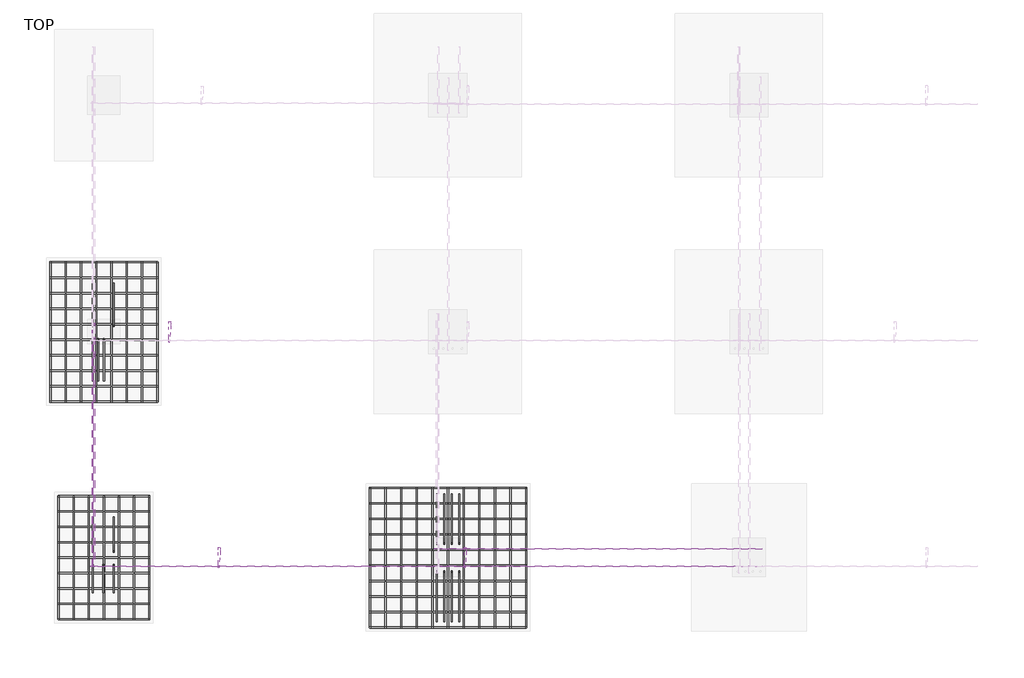
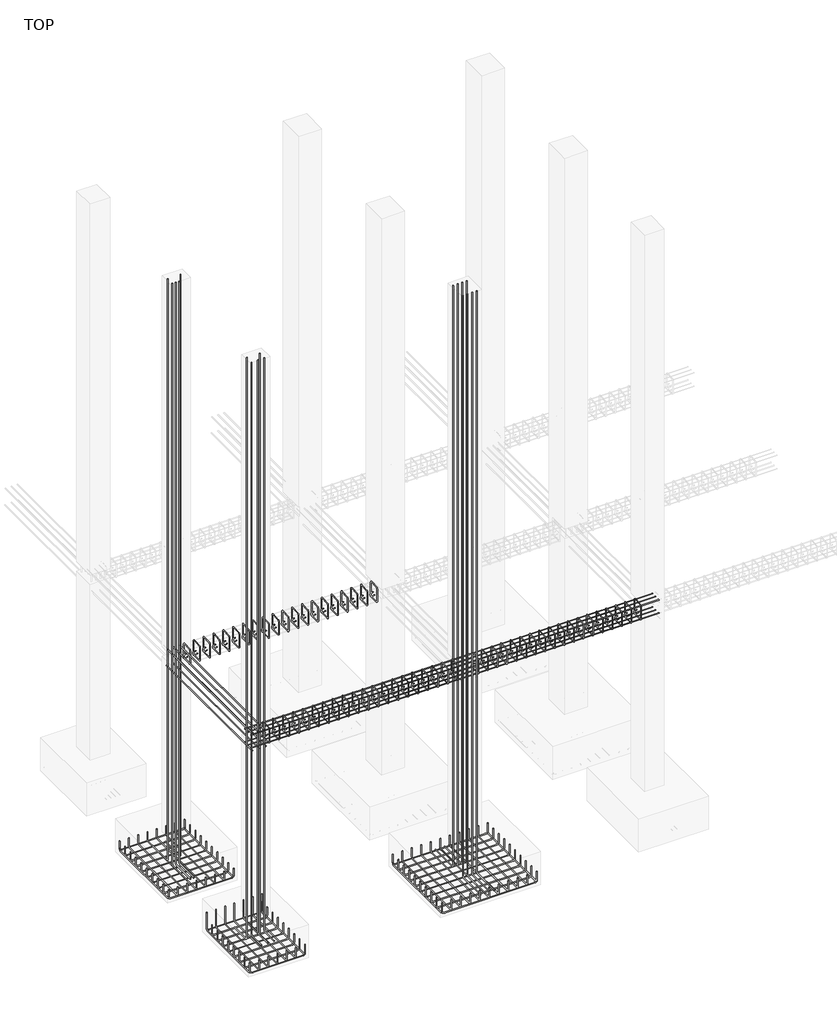
# One storey, part 2 of 8: 21 reinforcing bars.
"""IFC4 building model written with IfcOpenShell, lengths in millimetres."""

from ifc_helpers import new_model, si_unit, point, frame, origin, place, context, project, spatial, polyline, circle_curve, trimmed, segment, composite_curve, source, transform, mapped, element, save
from ifc_brep_helpers import swept_disk

model = new_model("IFC4")

# Units and contexts
model_context = context("Model", 3, world=origin())
ifc_project = project(units=[si_unit("LENGTHUNIT", "METRE", prefix="MILLI")], contexts=[model_context])

# Site, building, storey
site = spatial("IfcSite", under=ifc_project)
building = spatial("IfcBuilding", under=site)
storey = spatial("IfcBuildingStorey", under=building, Name="TOP", Elevation=0.0)

# Reinforcing bars
placement = place(None, origin())
reinforcing_bar_shape = source(origin(), model_context, "Body", "SolidModel", [
    swept_disk(composite_curve([segment(polyline([(-4743.7160601, 1689.3463601, -206.0605272), (-4743.7160601, 1689.3463601, -467.4)]), True, "CONTINUOUS"), segment(trimmed(circle_curve(frame((-4743.7160601, 1659.3463601, -467.4), z_axis=(-1.0, 0.0, 0.0), x_axis=(0.0, 30.0, 0.0)), 30.0), [point((-4743.7160601, 1689.3463601, -467.4))], [point((-4743.7160601, 1659.3463601, -497.4))], True, "CARTESIAN"), True, "CONTINUOUS"), segment(polyline([(-4743.7160601, 1659.3463601, -497.4), (-4743.7160601, 577.5307576, -497.4)]), True, "CONTINUOUS"), segment(trimmed(circle_curve(frame((-4743.7160601, 577.5307576, -467.4), z_axis=(-1.0, 0.0, 0.0), x_axis=(0.0, 0.0, -30.0)), 30.0), [point((-4743.7160601, 577.5307576, -497.4))], [point((-4743.7160601, 547.5307576, -467.4))], True, "CARTESIAN"), True, "CONTINUOUS"), segment(polyline([(-4743.7160601, 547.5307576, -467.4), (-4743.7160601, 547.5307576, -331.0)]), True, "CONTINUOUS")], self_intersect=False), 6.0),
])
element("IfcReinforcingBar", 1, at=placement, inside=storey, context=model_context, shape_type="MappedRepresentation", body=[
    mapped(reinforcing_bar_shape, transform((0.0, 0.0, 0.0), x_axis=(1.0, 0.0, 0.0), y_axis=(0.0, 1.0, 0.0), z_axis=(0.0, 0.0, 1.0))),
    mapped(reinforcing_bar_shape, transform((-140.4, 0.0, 0.0), x_axis=(1.0, 0.0, 0.0), y_axis=(0.0, 1.0, 0.0), z_axis=(0.0, 0.0, 1.0))),
    mapped(reinforcing_bar_shape, transform((-280.8, 0.0, 0.0), x_axis=(1.0, 0.0, 0.0), y_axis=(0.0, 1.0, 0.0), z_axis=(0.0, 0.0, 1.0))),
    mapped(reinforcing_bar_shape, transform((-421.2, 0.0, 0.0), x_axis=(1.0, 0.0, 0.0), y_axis=(0.0, 1.0, 0.0), z_axis=(0.0, 0.0, 1.0))),
    mapped(reinforcing_bar_shape, transform((-561.6, 0.0, 0.0), x_axis=(1.0, 0.0, 0.0), y_axis=(0.0, 1.0, 0.0), z_axis=(0.0, 0.0, 1.0))),
    mapped(reinforcing_bar_shape, transform((-702.0, 0.0, 0.0), x_axis=(1.0, 0.0, 0.0), y_axis=(0.0, 1.0, 0.0), z_axis=(0.0, 0.0, 1.0))),
    mapped(reinforcing_bar_shape, transform((-842.4, 0.0, 0.0), x_axis=(1.0, 0.0, 0.0), y_axis=(0.0, 1.0, 0.0), z_axis=(0.0, 0.0, 1.0))),
])
reinforcing_bar_2_shape = source(origin(), model_context, "Body", "SolidModel", [
    swept_disk(composite_curve([segment(polyline([(-5586.1160601, 1694.7307576, -331.0), (-5586.1160601, 1694.7307576, -467.4)]), True, "CONTINUOUS"), segment(trimmed(circle_curve(frame((-5556.1160601, 1694.7307576, -467.4), z_axis=(0.0, -1.0, 0.0), x_axis=(-30.0, 0.0, 0.0)), 30.0), [point((-5586.1160601, 1694.7307576, -467.4))], [point((-5556.1160601, 1694.7307576, -497.4))], True, "CARTESIAN"), True, "CONTINUOUS"), segment(polyline([(-5556.1160601, 1694.7307576, -497.4), (-4773.7160601, 1694.7307576, -497.4)]), True, "CONTINUOUS"), segment(trimmed(circle_curve(frame((-4773.7160601, 1694.7307576, -467.4), z_axis=(0.0, -1.0, 0.0), x_axis=(0.0, 0.0, -30.0)), 30.0), [point((-4773.7160601, 1694.7307576, -497.4))], [point((-4743.7160601, 1694.7307576, -467.4))], True, "CARTESIAN"), True, "CONTINUOUS"), segment(polyline([(-4743.7160601, 1694.7307576, -467.4), (-4743.7160601, 1694.7307576, -331.0)]), True, "CONTINUOUS")], self_intersect=False), 6.0),
])
element("IfcReinforcingBar", 2, at=placement, inside=storey, context=model_context, shape_type="MappedRepresentation", body=[
    mapped(reinforcing_bar_2_shape, transform((0.0, 0.0, 0.0), x_axis=(1.0, 0.0, 0.0), y_axis=(0.0, 1.0, 0.0), z_axis=(0.0, 0.0, 1.0))),
    mapped(reinforcing_bar_2_shape, transform((0.0, -143.4, 0.0), x_axis=(1.0, 0.0, 0.0), y_axis=(0.0, 1.0, 0.0), z_axis=(0.0, 0.0, 1.0))),
    mapped(reinforcing_bar_2_shape, transform((0.0, -286.8, 0.0), x_axis=(1.0, 0.0, 0.0), y_axis=(0.0, 1.0, 0.0), z_axis=(0.0, 0.0, 1.0))),
    mapped(reinforcing_bar_2_shape, transform((0.0, -430.2, 0.0), x_axis=(1.0, 0.0, 0.0), y_axis=(0.0, 1.0, 0.0), z_axis=(0.0, 0.0, 1.0))),
    mapped(reinforcing_bar_2_shape, transform((0.0, -573.6, 0.0), x_axis=(1.0, 0.0, 0.0), y_axis=(0.0, 1.0, 0.0), z_axis=(0.0, 0.0, 1.0))),
    mapped(reinforcing_bar_2_shape, transform((0.0, -717.0, 0.0), x_axis=(1.0, 0.0, 0.0), y_axis=(0.0, 1.0, 0.0), z_axis=(0.0, 0.0, 1.0))),
    mapped(reinforcing_bar_2_shape, transform((0.0, -860.4, 0.0), x_axis=(1.0, 0.0, 0.0), y_axis=(0.0, 1.0, 0.0), z_axis=(0.0, 0.0, 1.0))),
    mapped(reinforcing_bar_2_shape, transform((0.0, -1003.8, 0.0), x_axis=(1.0, 0.0, 0.0), y_axis=(0.0, 1.0, 0.0), z_axis=(0.0, 0.0, 1.0))),
    mapped(reinforcing_bar_2_shape, transform((0.0, -1147.2, 0.0), x_axis=(1.0, 0.0, 0.0), y_axis=(0.0, 1.0, 0.0), z_axis=(0.0, 0.0, 1.0))),
])
reinforcing_bar_3_shape = source(origin(), model_context, "Body", "SolidModel", [
    swept_disk(composite_curve([segment(polyline([(-5269.3160601, 1177.1568407, 8968.464), (-5269.3160601, 1177.1568407, -415.886)]), True, "CONTINUOUS"), segment(trimmed(circle_curve(frame((-5269.3160601, 1207.1568407, -415.886), z_axis=(1.0, 0.0, 0.0), x_axis=(0.0, -30.0, 0.0)), 30.0), [point((-5269.3160601, 1177.1568407, -415.886))], [point((-5269.3160601, 1207.1568407, -445.886))], True, "CARTESIAN"), True, "CONTINUOUS"), segment(polyline([(-5269.3160601, 1207.1568407, -445.886), (-5269.3160601, 1500.2307576, -445.886)]), True, "CONTINUOUS")], self_intersect=False), 6.0),
])
element("IfcReinforcingBar", 3, at=placement, inside=storey, context=model_context, shape_type="MappedRepresentation", body=[
    mapped(reinforcing_bar_3_shape, transform((0.0, 0.0, 0.0), x_axis=(1.0, 0.0, 0.0), y_axis=(0.0, 1.0, 0.0), z_axis=(0.0, 0.0, 1.0))),
    mapped(reinforcing_bar_3_shape, transform((195.9681172, 0.0, 0.0), x_axis=(1.0, 0.0, 0.0), y_axis=(0.0, 1.0, 0.0), z_axis=(0.0, 0.0, 1.0))),
])
reinforcing_bar_4_shape = source(origin(), model_context, "Body", "SolidModel", [
    swept_disk(composite_curve([segment(polyline([(-5073.3479429, 1054.8307576, 8968.464), (-5073.3479429, 1054.8307576, -276.4542625)]), True, "CONTINUOUS"), segment(trimmed(circle_curve(frame((-5073.3479429, 1024.8307576, -276.4542625), z_axis=(-1.0, 0.0, 0.0), x_axis=(0.0, 30.0, 0.0)), 30.0), [point((-5073.3479429, 1054.8307576, -276.4542625))], [point((-5073.3479429, 1024.8307576, -306.4542625))], True, "CARTESIAN"), True, "CONTINUOUS"), segment(polyline([(-5073.3479429, 1024.8307576, -306.4542625), (-5073.3479429, 793.417504, -306.4542625)]), True, "CONTINUOUS")], self_intersect=False), 6.0),
])
element("IfcReinforcingBar", 4, at=placement, inside=storey, context=model_context, shape_type="MappedRepresentation", body=[
    mapped(reinforcing_bar_4_shape, transform((0.0, 0.0, 0.0), x_axis=(1.0, 0.0, 0.0), y_axis=(0.0, 1.0, 0.0), z_axis=(0.0, 0.0, 1.0))),
    mapped(reinforcing_bar_4_shape, transform((-97.9840586, 0.0, 0.0), x_axis=(1.0, 0.0, 0.0), y_axis=(0.0, 1.0, 0.0), z_axis=(0.0, 0.0, 1.0))),
    mapped(reinforcing_bar_4_shape, transform((-195.9681172, 0.0, 0.0), x_axis=(1.0, 0.0, 0.0), y_axis=(0.0, 1.0, 0.0), z_axis=(0.0, 0.0, 1.0))),
])
reinforcing_bar_5_shape = source(origin(), model_context, "Body", "SolidModel", [
    swept_disk(composite_curve([segment(polyline([(-5269.3160601, 3277.1568407, 8968.464), (-5269.3160601, 3277.1568407, -415.886)]), True, "CONTINUOUS"), segment(trimmed(circle_curve(frame((-5269.3160601, 3307.1568407, -415.886), z_axis=(1.0, 0.0, 0.0), x_axis=(0.0, -30.0, 0.0)), 30.0), [point((-5269.3160601, 3277.1568407, -415.886))], [point((-5269.3160601, 3307.1568407, -445.886))], True, "CARTESIAN"), True, "CONTINUOUS"), segment(polyline([(-5269.3160601, 3307.1568407, -445.886), (-5269.3160601, 3676.4307576, -445.886)]), True, "CONTINUOUS")], self_intersect=False), 6.0),
])
element("IfcReinforcingBar", 5, at=placement, inside=storey, context=model_context, shape_type="MappedRepresentation", body=[
    mapped(reinforcing_bar_5_shape, transform((0.0, 0.0, 0.0), x_axis=(1.0, 0.0, 0.0), y_axis=(0.0, 1.0, 0.0), z_axis=(0.0, 0.0, 1.0))),
    mapped(reinforcing_bar_5_shape, transform((195.9681172, 0.0, 0.0), x_axis=(1.0, 0.0, 0.0), y_axis=(0.0, 1.0, 0.0), z_axis=(0.0, 0.0, 1.0))),
])
reinforcing_bar_6_shape = source(origin(), model_context, "Body", "SolidModel", [
    swept_disk(composite_curve([segment(polyline([(-5164.9160601, 3154.8307576, 8968.464), (-5164.9160601, 3154.8307576, -415.886)]), True, "CONTINUOUS"), segment(trimmed(circle_curve(frame((-5164.9160601, 3124.8307576, -415.886), z_axis=(-1.0, 0.0, 0.0), x_axis=(0.0, 30.0, 0.0)), 30.0), [point((-5164.9160601, 3154.8307576, -415.886))], [point((-5164.9160601, 3124.8307576, -445.886))], True, "CARTESIAN"), True, "CONTINUOUS"), segment(polyline([(-5164.9160601, 3124.8307576, -445.886), (-5164.9160601, 2765.8307576, -445.886)]), True, "CONTINUOUS")], self_intersect=False), 6.0),
])
element("IfcReinforcingBar", 6, at=placement, inside=storey, context=model_context, shape_type="MappedRepresentation", body=[
    mapped(reinforcing_bar_6_shape, transform((0.0, 0.0, 0.0), x_axis=(1.0, 0.0, 0.0), y_axis=(0.0, 1.0, 0.0), z_axis=(0.0, 0.0, 1.0))),
    mapped(reinforcing_bar_6_shape, transform((-52.2, 0.0, 0.0), x_axis=(1.0, 0.0, 0.0), y_axis=(0.0, 1.0, 0.0), z_axis=(0.0, 0.0, 1.0))),
    mapped(reinforcing_bar_6_shape, transform((-104.4, 0.0, 0.0), x_axis=(1.0, 0.0, 0.0), y_axis=(0.0, 1.0, 0.0), z_axis=(0.0, 0.0, 1.0))),
])
reinforcing_bar_7_shape = source(origin(), model_context, "Body", "SolidModel", [
    swept_disk(composite_curve([segment(polyline([(-2069.3160601, 1250.9815576, 8968.464), (-2069.3160601, 1250.9815576, -409.536)]), True, "CONTINUOUS"), segment(trimmed(circle_curve(frame((-2069.3160601, 1280.9815576, -409.536), z_axis=(1.0, 0.0, 0.0), x_axis=(0.0, -30.0, 0.0)), 30.0), [point((-2069.3160601, 1250.9815576, -409.536))], [point((-2069.3160601, 1280.9815576, -439.536))], True, "CARTESIAN"), True, "CONTINUOUS"), segment(polyline([(-2069.3160601, 1280.9815576, -439.536), (-2069.3160601, 1716.1815576, -439.536)]), True, "CONTINUOUS")], self_intersect=False), 6.0),
])
element("IfcReinforcingBar", 7, at=placement, inside=storey, context=model_context, shape_type="MappedRepresentation", body=[
    mapped(reinforcing_bar_7_shape, transform((0.0, 0.0, 0.0), x_axis=(1.0, 0.0, 0.0), y_axis=(0.0, 1.0, 0.0), z_axis=(0.0, 0.0, 1.0))),
    mapped(reinforcing_bar_7_shape, transform((69.6, 0.0, 0.0), x_axis=(1.0, 0.0, 0.0), y_axis=(0.0, 1.0, 0.0), z_axis=(0.0, 0.0, 1.0))),
    mapped(reinforcing_bar_7_shape, transform((139.2, 0.0, 0.0), x_axis=(1.0, 0.0, 0.0), y_axis=(0.0, 1.0, 0.0), z_axis=(0.0, 0.0, 1.0))),
    mapped(reinforcing_bar_7_shape, transform((208.8, 0.0, 0.0), x_axis=(1.0, 0.0, 0.0), y_axis=(0.0, 1.0, 0.0), z_axis=(0.0, 0.0, 1.0))),
])
reinforcing_bar_8_shape = source(origin(), model_context, "Body", "SolidModel", [
    swept_disk(composite_curve([segment(polyline([(-1860.5160601, 991.2799576, 8968.464), (-1860.5160601, 991.2799576, -415.886)]), True, "CONTINUOUS"), segment(trimmed(circle_curve(frame((-1860.5160601, 961.2799576, -415.886), z_axis=(-1.0, 0.0, 0.0), x_axis=(0.0, 30.0, 0.0)), 30.0), [point((-1860.5160601, 991.2799576, -415.886))], [point((-1860.5160601, 961.2799576, -445.886))], True, "CARTESIAN"), True, "CONTINUOUS"), segment(polyline([(-1860.5160601, 961.2799576, -445.886), (-1860.5160601, 526.0799576, -445.886)]), True, "CONTINUOUS")], self_intersect=False), 6.0),
])
element("IfcReinforcingBar", 8, at=placement, inside=storey, context=model_context, shape_type="MappedRepresentation", body=[
    mapped(reinforcing_bar_8_shape, transform((0.0, 0.0, 0.0), x_axis=(1.0, 0.0, 0.0), y_axis=(0.0, 1.0, 0.0), z_axis=(0.0, 0.0, 1.0))),
    mapped(reinforcing_bar_8_shape, transform((-69.6, 0.0, 0.0), x_axis=(1.0, 0.0, 0.0), y_axis=(0.0, 1.0, 0.0), z_axis=(0.0, 0.0, 1.0))),
    mapped(reinforcing_bar_8_shape, transform((-139.2, 0.0, 0.0), x_axis=(1.0, 0.0, 0.0), y_axis=(0.0, 1.0, 0.0), z_axis=(0.0, 0.0, 1.0))),
    mapped(reinforcing_bar_8_shape, transform((-208.8, 0.0, 0.0), x_axis=(1.0, 0.0, 0.0), y_axis=(0.0, 1.0, 0.0), z_axis=(0.0, 0.0, 1.0))),
])
reinforcing_bar_9_shape = source(origin(), model_context, "Body", "SolidModel", [
    swept_disk(composite_curve([segment(polyline([(-4667.5160601, 3870.9307576, -351.0), (-4667.5160601, 3870.9307576, -467.4)]), True, "CONTINUOUS"), segment(trimmed(circle_curve(frame((-4667.5160601, 3840.9307576, -467.4), z_axis=(-1.0, 0.0, 0.0), x_axis=(0.0, 30.0, 0.0)), 30.0), [point((-4667.5160601, 3870.9307576, -467.4))], [point((-4667.5160601, 3840.9307576, -497.4))], True, "CARTESIAN"), True, "CONTINUOUS"), segment(polyline([(-4667.5160601, 3840.9307576, -497.4), (-4667.5160601, 2601.3307576, -497.4)]), True, "CONTINUOUS"), segment(trimmed(circle_curve(frame((-4667.5160601, 2601.3307576, -467.4), z_axis=(-1.0, 0.0, 0.0), x_axis=(0.0, 0.0, -30.0)), 30.0), [point((-4667.5160601, 2601.3307576, -497.4))], [point((-4667.5160601, 2571.3307576, -467.4))], True, "CARTESIAN"), True, "CONTINUOUS"), segment(polyline([(-4667.5160601, 2571.3307576, -467.4), (-4667.5160601, 2571.3307576, -351.0)]), True, "CONTINUOUS")], self_intersect=False), 6.0),
])
element("IfcReinforcingBar", 9, at=placement, inside=storey, context=model_context, shape_type="MappedRepresentation", body=[
    mapped(reinforcing_bar_9_shape, transform((0.0, 0.0, 0.0), x_axis=(1.0, 0.0, 0.0), y_axis=(0.0, 1.0, 0.0), z_axis=(0.0, 0.0, 1.0))),
    mapped(reinforcing_bar_9_shape, transform((-142.1142857, 0.0, 0.0), x_axis=(1.0, 0.0, 0.0), y_axis=(0.0, 1.0, 0.0), z_axis=(0.0, 0.0, 1.0))),
    mapped(reinforcing_bar_9_shape, transform((-284.2285714, 0.0, 0.0), x_axis=(1.0, 0.0, 0.0), y_axis=(0.0, 1.0, 0.0), z_axis=(0.0, 0.0, 1.0))),
    mapped(reinforcing_bar_9_shape, transform((-426.3428571, 0.0, 0.0), x_axis=(1.0, 0.0, 0.0), y_axis=(0.0, 1.0, 0.0), z_axis=(0.0, 0.0, 1.0))),
    mapped(reinforcing_bar_9_shape, transform((-568.4571429, 0.0, 0.0), x_axis=(1.0, 0.0, 0.0), y_axis=(0.0, 1.0, 0.0), z_axis=(0.0, 0.0, 1.0))),
    mapped(reinforcing_bar_9_shape, transform((-710.5714286, 0.0, 0.0), x_axis=(1.0, 0.0, 0.0), y_axis=(0.0, 1.0, 0.0), z_axis=(0.0, 0.0, 1.0))),
    mapped(reinforcing_bar_9_shape, transform((-852.6857143, 0.0, 0.0), x_axis=(1.0, 0.0, 0.0), y_axis=(0.0, 1.0, 0.0), z_axis=(0.0, 0.0, 1.0))),
    mapped(reinforcing_bar_9_shape, transform((-994.8, 0.0, 0.0), x_axis=(1.0, 0.0, 0.0), y_axis=(0.0, 1.0, 0.0), z_axis=(0.0, 0.0, 1.0))),
])
reinforcing_bar_10_shape = source(origin(), model_context, "Body", "SolidModel", [
    swept_disk(composite_curve([segment(polyline([(-5662.3160601, 3870.9307576, -351.0), (-5662.3160601, 3870.9307576, -467.4)]), True, "CONTINUOUS"), segment(trimmed(circle_curve(frame((-5632.3160601, 3870.9307576, -467.4), z_axis=(0.0, -1.0, 0.0), x_axis=(-30.0, 0.0, 0.0)), 30.0), [point((-5662.3160601, 3870.9307576, -467.4))], [point((-5632.3160601, 3870.9307576, -497.4))], True, "CARTESIAN"), True, "CONTINUOUS"), segment(polyline([(-5632.3160601, 3870.9307576, -497.4), (-4697.5160601, 3870.9307576, -497.4)]), True, "CONTINUOUS"), segment(trimmed(circle_curve(frame((-4697.5160601, 3870.9307576, -467.4), z_axis=(0.0, -1.0, 0.0), x_axis=(0.0, 0.0, -30.0)), 30.0), [point((-4697.5160601, 3870.9307576, -497.4))], [point((-4667.5160601, 3870.9307576, -467.4))], True, "CARTESIAN"), True, "CONTINUOUS"), segment(polyline([(-4667.5160601, 3870.9307576, -467.4), (-4667.5160601, 3870.9307576, -351.0)]), True, "CONTINUOUS")], self_intersect=False), 6.0),
])
element("IfcReinforcingBar", 10, at=placement, inside=storey, context=model_context, shape_type="MappedRepresentation", body=[
    mapped(reinforcing_bar_10_shape, transform((0.0, 0.0, 0.0), x_axis=(1.0, 0.0, 0.0), y_axis=(0.0, 1.0, 0.0), z_axis=(0.0, 0.0, 1.0))),
    mapped(reinforcing_bar_10_shape, transform((0.0, -144.4, 0.0), x_axis=(1.0, 0.0, 0.0), y_axis=(0.0, 1.0, 0.0), z_axis=(0.0, 0.0, 1.0))),
    mapped(reinforcing_bar_10_shape, transform((0.0, -288.8, 0.0), x_axis=(1.0, 0.0, 0.0), y_axis=(0.0, 1.0, 0.0), z_axis=(0.0, 0.0, 1.0))),
    mapped(reinforcing_bar_10_shape, transform((0.0, -433.2, 0.0), x_axis=(1.0, 0.0, 0.0), y_axis=(0.0, 1.0, 0.0), z_axis=(0.0, 0.0, 1.0))),
    mapped(reinforcing_bar_10_shape, transform((0.0, -577.6, 0.0), x_axis=(1.0, 0.0, 0.0), y_axis=(0.0, 1.0, 0.0), z_axis=(0.0, 0.0, 1.0))),
    mapped(reinforcing_bar_10_shape, transform((0.0, -722.0, 0.0), x_axis=(1.0, 0.0, 0.0), y_axis=(0.0, 1.0, 0.0), z_axis=(0.0, 0.0, 1.0))),
    mapped(reinforcing_bar_10_shape, transform((0.0, -866.4, 0.0), x_axis=(1.0, 0.0, 0.0), y_axis=(0.0, 1.0, 0.0), z_axis=(0.0, 0.0, 1.0))),
    mapped(reinforcing_bar_10_shape, transform((0.0, -1010.8, 0.0), x_axis=(1.0, 0.0, 0.0), y_axis=(0.0, 1.0, 0.0), z_axis=(0.0, 0.0, 1.0))),
    mapped(reinforcing_bar_10_shape, transform((0.0, -1155.2, 0.0), x_axis=(1.0, 0.0, 0.0), y_axis=(0.0, 1.0, 0.0), z_axis=(0.0, 0.0, 1.0))),
    mapped(reinforcing_bar_10_shape, transform((0.0, -1299.6, 0.0), x_axis=(1.0, 0.0, 0.0), y_axis=(0.0, 1.0, 0.0), z_axis=(0.0, 0.0, 1.0))),
])
reinforcing_bar_11_shape = source(origin(), model_context, "Body", "SolidModel", [
    swept_disk(composite_curve([segment(polyline([(-2690.9160601, 471.3307576, -331.0), (-2690.9160601, 471.3307576, -467.4)]), True, "CONTINUOUS"), segment(trimmed(circle_curve(frame((-2690.9160601, 501.3307576, -467.4), z_axis=(1.0, 0.0, 0.0), x_axis=(0.0, -30.0, 0.0)), 30.0), [point((-2690.9160601, 471.3307576, -467.4))], [point((-2690.9160601, 501.3307576, -497.4))], True, "CARTESIAN"), True, "CONTINUOUS"), segment(polyline([(-2690.9160601, 501.3307576, -497.4), (-2690.9160601, 1740.9307576, -497.4)]), True, "CONTINUOUS"), segment(trimmed(circle_curve(frame((-2690.9160601, 1740.9307576, -467.4), z_axis=(1.0, 0.0, 0.0), x_axis=(0.0, 0.0, -30.0)), 30.0), [point((-2690.9160601, 1740.9307576, -497.4))], [point((-2690.9160601, 1770.9307576, -467.4))], True, "CARTESIAN"), True, "CONTINUOUS"), segment(polyline([(-2690.9160601, 1770.9307576, -467.4), (-2690.9160601, 1770.9307576, -331.0)]), True, "CONTINUOUS")], self_intersect=False), 6.0),
])
element("IfcReinforcingBar", 11, at=placement, inside=storey, context=model_context, shape_type="MappedRepresentation", body=[
    mapped(reinforcing_bar_11_shape, transform((0.0, 0.0, 0.0), x_axis=(1.0, 0.0, 0.0), y_axis=(0.0, 1.0, 0.0), z_axis=(0.0, 0.0, 1.0))),
    mapped(reinforcing_bar_11_shape, transform((145.2, 0.0, 0.0), x_axis=(1.0, 0.0, 0.0), y_axis=(0.0, 1.0, 0.0), z_axis=(0.0, 0.0, 1.0))),
    mapped(reinforcing_bar_11_shape, transform((290.4, 0.0, 0.0), x_axis=(1.0, 0.0, 0.0), y_axis=(0.0, 1.0, 0.0), z_axis=(0.0, 0.0, 1.0))),
    mapped(reinforcing_bar_11_shape, transform((435.6, 0.0, 0.0), x_axis=(1.0, 0.0, 0.0), y_axis=(0.0, 1.0, 0.0), z_axis=(0.0, 0.0, 1.0))),
    mapped(reinforcing_bar_11_shape, transform((580.8, 0.0, 0.0), x_axis=(1.0, 0.0, 0.0), y_axis=(0.0, 1.0, 0.0), z_axis=(0.0, 0.0, 1.0))),
    mapped(reinforcing_bar_11_shape, transform((726.0, 0.0, 0.0), x_axis=(1.0, 0.0, 0.0), y_axis=(0.0, 1.0, 0.0), z_axis=(0.0, 0.0, 1.0))),
    mapped(reinforcing_bar_11_shape, transform((871.2, 0.0, 0.0), x_axis=(1.0, 0.0, 0.0), y_axis=(0.0, 1.0, 0.0), z_axis=(0.0, 0.0, 1.0))),
    mapped(reinforcing_bar_11_shape, transform((1016.4, 0.0, 0.0), x_axis=(1.0, 0.0, 0.0), y_axis=(0.0, 1.0, 0.0), z_axis=(0.0, 0.0, 1.0))),
    mapped(reinforcing_bar_11_shape, transform((1161.6, 0.0, 0.0), x_axis=(1.0, 0.0, 0.0), y_axis=(0.0, 1.0, 0.0), z_axis=(0.0, 0.0, 1.0))),
    mapped(reinforcing_bar_11_shape, transform((1306.8, 0.0, 0.0), x_axis=(1.0, 0.0, 0.0), y_axis=(0.0, 1.0, 0.0), z_axis=(0.0, 0.0, 1.0))),
    mapped(reinforcing_bar_11_shape, transform((1452.0, 0.0, 0.0), x_axis=(1.0, 0.0, 0.0), y_axis=(0.0, 1.0, 0.0), z_axis=(0.0, 0.0, 1.0))),
])
reinforcing_bar_12_shape = source(origin(), model_context, "Body", "SolidModel", [
    swept_disk(composite_curve([segment(polyline([(-1238.9160601, 471.3307576, -331.0), (-1238.9160601, 471.3307576, -467.4)]), True, "CONTINUOUS"), segment(trimmed(circle_curve(frame((-1268.9160601, 471.3307576, -467.4), z_axis=(0.0, 1.0, 0.0), x_axis=(30.0, 0.0, 0.0)), 30.0), [point((-1238.9160601, 471.3307576, -467.4))], [point((-1268.9160601, 471.3307576, -497.4))], True, "CARTESIAN"), True, "CONTINUOUS"), segment(polyline([(-1268.9160601, 471.3307576, -497.4), (-2660.9160601, 471.3307576, -497.4)]), True, "CONTINUOUS"), segment(trimmed(circle_curve(frame((-2660.9160601, 471.3307576, -467.4), z_axis=(0.0, 1.0, 0.0), x_axis=(0.0, 0.0, -30.0)), 30.0), [point((-2660.9160601, 471.3307576, -497.4))], [point((-2690.9160601, 471.3307576, -467.4))], True, "CARTESIAN"), True, "CONTINUOUS"), segment(polyline([(-2690.9160601, 471.3307576, -467.4), (-2690.9160601, 471.3307576, -331.0)]), True, "CONTINUOUS")], self_intersect=False), 6.0),
])
element("IfcReinforcingBar", 12, at=placement, inside=storey, context=model_context, shape_type="MappedRepresentation", body=[
    mapped(reinforcing_bar_12_shape, transform((0.0, 0.0, 0.0), x_axis=(1.0, 0.0, 0.0), y_axis=(0.0, 1.0, 0.0), z_axis=(0.0, 0.0, 1.0))),
    mapped(reinforcing_bar_12_shape, transform((0.0, 144.4, 0.0), x_axis=(1.0, 0.0, 0.0), y_axis=(0.0, 1.0, 0.0), z_axis=(0.0, 0.0, 1.0))),
    mapped(reinforcing_bar_12_shape, transform((0.0, 288.8, 0.0), x_axis=(1.0, 0.0, 0.0), y_axis=(0.0, 1.0, 0.0), z_axis=(0.0, 0.0, 1.0))),
    mapped(reinforcing_bar_12_shape, transform((0.0, 433.2, 0.0), x_axis=(1.0, 0.0, 0.0), y_axis=(0.0, 1.0, 0.0), z_axis=(0.0, 0.0, 1.0))),
    mapped(reinforcing_bar_12_shape, transform((0.0, 577.6, 0.0), x_axis=(1.0, 0.0, 0.0), y_axis=(0.0, 1.0, 0.0), z_axis=(0.0, 0.0, 1.0))),
    mapped(reinforcing_bar_12_shape, transform((0.0, 722.0, 0.0), x_axis=(1.0, 0.0, 0.0), y_axis=(0.0, 1.0, 0.0), z_axis=(0.0, 0.0, 1.0))),
    mapped(reinforcing_bar_12_shape, transform((0.0, 866.4, 0.0), x_axis=(1.0, 0.0, 0.0), y_axis=(0.0, 1.0, 0.0), z_axis=(0.0, 0.0, 1.0))),
    mapped(reinforcing_bar_12_shape, transform((0.0, 1010.8, 0.0), x_axis=(1.0, 0.0, 0.0), y_axis=(0.0, 1.0, 0.0), z_axis=(0.0, 0.0, 1.0))),
    mapped(reinforcing_bar_12_shape, transform((0.0, 1155.2, 0.0), x_axis=(1.0, 0.0, 0.0), y_axis=(0.0, 1.0, 0.0), z_axis=(0.0, 0.0, 1.0))),
    mapped(reinforcing_bar_12_shape, transform((0.0, 1299.6, 0.0), x_axis=(1.0, 0.0, 0.0), y_axis=(0.0, 1.0, 0.0), z_axis=(0.0, 0.0, 1.0))),
])
reinforcing_bar_13_shape = source(origin(), model_context, "Body", "SolidModel", [
    swept_disk(composite_curve([segment(polyline([(-5267.9226618, 3305.4307576, 2693.6917983), (-5267.9226618, 1036.8307576, 2693.6917983)]), True, "CONTINUOUS")], self_intersect=False), 5.0),
])
element("IfcReinforcingBar", 13, at=placement, inside=storey, context=model_context, shape_type="MappedRepresentation", body=[
    mapped(reinforcing_bar_13_shape, transform((0.0, 0.0, 0.0), x_axis=(1.0, 0.0, 0.0), y_axis=(0.0, 1.0, 0.0), z_axis=(0.0, 0.0, 1.0))),
    mapped(reinforcing_bar_13_shape, transform((103.0066017, 0.0, 0.0), x_axis=(1.0, 0.0, 0.0), y_axis=(0.0, 1.0, 0.0), z_axis=(0.0, 0.0, 1.0))),
    mapped(reinforcing_bar_13_shape, transform((206.0132034, 0.0, 0.0), x_axis=(1.0, 0.0, 0.0), y_axis=(0.0, 1.0, 0.0), z_axis=(0.0, 0.0, 1.0))),
])
reinforcing_bar_14_shape = source(origin(), model_context, "Body", "SolidModel", [
    swept_disk(composite_curve([segment(polyline([(-5257.3160601, 1036.8307576, 2955.0), (-5257.3160601, 3305.4307576, 2955.0)]), True, "CONTINUOUS")], self_intersect=False), 5.0),
])
element("IfcReinforcingBar", 14, at=placement, inside=storey, context=model_context, shape_type="MappedRepresentation", body=[
    mapped(reinforcing_bar_14_shape, transform((0.0, 0.0, 0.0), x_axis=(1.0, 0.0, 0.0), y_axis=(0.0, 1.0, 0.0), z_axis=(0.0, 0.0, 1.0))),
    mapped(reinforcing_bar_14_shape, transform((92.4, 0.0, 0.0), x_axis=(1.0, 0.0, 0.0), y_axis=(0.0, 1.0, 0.0), z_axis=(0.0, 0.0, 1.0))),
    mapped(reinforcing_bar_14_shape, transform((184.8, 0.0, 0.0), x_axis=(1.0, 0.0, 0.0), y_axis=(0.0, 1.0, 0.0), z_axis=(0.0, 0.0, 1.0))),
])
reinforcing_bar_15_shape = source(origin(), model_context, "Body", "SolidModel", [
    swept_disk(composite_curve([segment(polyline([(-2121.7668601, 1143.8753761, 2827.6888527), (-2121.7668601, 1208.2220932, 2763.3421356)]), True, "CONTINUOUS"), segment(trimmed(circle_curve(frame((-2121.7668601, 1194.0799576, 2749.2), z_axis=(-1.0, 0.0, 0.0), x_axis=(0.0, 14.142135600000074, 14.142135600000074)), 20.0), [point((-2121.7668601, 1208.2220932, 2763.3421356))], [point((-2121.7668601, 1194.0799576, 2729.2))], True, "CARTESIAN"), True, "CONTINUOUS"), segment(polyline([(-2121.7668601, 1194.0799576, 2729.2), (-2121.7668601, 1048.1815576, 2729.2)]), True, "CONTINUOUS"), segment(trimmed(circle_curve(frame((-2121.7668601, 1048.1815576, 2749.2), z_axis=(-1.0, 0.0, 0.0), x_axis=(0.0, 0.0, -20.0)), 20.0), [point((-2121.7668601, 1048.1815576, 2729.2))], [point((-2121.7668601, 1028.1815576, 2749.2))], True, "CARTESIAN"), True, "CONTINUOUS"), segment(polyline([(-2121.7668601, 1028.1815576, 2749.2), (-2121.7668601, 1028.1815576, 2946.0)]), True, "CONTINUOUS"), segment(trimmed(circle_curve(frame((-2120.9069707, 1048.1630638, 2946.0), z_axis=(-0.9990753104108542, 0.04299446624224495, 0.0), x_axis=(-0.8598894000001565, -19.981506200000013, 0.0)), 20.0), [point((-2121.7668601, 1028.1815576, 2946.0))], [point((-2120.9069707, 1048.1630638, 2966.0))], True, "CARTESIAN"), True, "CONTINUOUS"), segment(polyline([(-2120.9069707, 1048.1630638, 2966.0), (-2114.6267494, 1194.0984514, 2966.0)]), True, "CONTINUOUS"), segment(trimmed(circle_curve(frame((-2114.6267494, 1194.0984514, 2946.0), z_axis=(-0.9990753104108542, 0.04299446624224495, 0.0), x_axis=(0.0, 0.0, 20.0)), 20.0), [point((-2114.6267494, 1194.0984514, 2966.0))], [point((-2113.7668601, 1214.0799576, 2946.0))], True, "CARTESIAN"), True, "CONTINUOUS"), segment(polyline([(-2113.7668601, 1214.0799576, 2946.0), (-2113.7668601, 1214.0799576, 2749.2)]), True, "CONTINUOUS"), segment(trimmed(circle_curve(frame((-2113.7668601, 1194.0799576, 2749.2), z_axis=(-1.0, 0.0, 0.0), x_axis=(0.0, 20.0, 0.0)), 20.0), [point((-2113.7668601, 1214.0799576, 2749.2))], [point((-2113.7668601, 1179.937822, 2735.0578644))], True, "CARTESIAN"), True, "CONTINUOUS"), segment(polyline([(-2113.7668601, 1179.937822, 2735.0578644), (-2113.7668601, 1115.5911049, 2799.4045815)]), True, "CONTINUOUS")], self_intersect=False), 4.0),
])
element("IfcReinforcingBar", 15, at=placement, inside=storey, context=model_context, shape_type="MappedRepresentation", body=[
    mapped(reinforcing_bar_15_shape, transform((0.0, 0.0, 0.0), x_axis=(1.0, 0.0, 0.0), y_axis=(0.0, 1.0, 0.0), z_axis=(0.0, 0.0, 1.0))),
    mapped(reinforcing_bar_15_shape, transform((-151.9657474, 0.0, 0.0), x_axis=(1.0, 0.0, 0.0), y_axis=(0.0, 1.0, 0.0), z_axis=(0.0, 0.0, 1.0))),
    mapped(reinforcing_bar_15_shape, transform((-303.9314947, 0.0, 0.0), x_axis=(1.0, 0.0, 0.0), y_axis=(0.0, 1.0, 0.0), z_axis=(0.0, 0.0, 1.0))),
    mapped(reinforcing_bar_15_shape, transform((-455.8972421, 0.0, 0.0), x_axis=(1.0, 0.0, 0.0), y_axis=(0.0, 1.0, 0.0), z_axis=(0.0, 0.0, 1.0))),
    mapped(reinforcing_bar_15_shape, transform((-607.8629895, 0.0, 0.0), x_axis=(1.0, 0.0, 0.0), y_axis=(0.0, 1.0, 0.0), z_axis=(0.0, 0.0, 1.0))),
    mapped(reinforcing_bar_15_shape, transform((-759.8287368, 0.0, 0.0), x_axis=(1.0, 0.0, 0.0), y_axis=(0.0, 1.0, 0.0), z_axis=(0.0, 0.0, 1.0))),
    mapped(reinforcing_bar_15_shape, transform((-911.7944842, 0.0, 0.0), x_axis=(1.0, 0.0, 0.0), y_axis=(0.0, 1.0, 0.0), z_axis=(0.0, 0.0, 1.0))),
    mapped(reinforcing_bar_15_shape, transform((-1063.7602316, 0.0, 0.0), x_axis=(1.0, 0.0, 0.0), y_axis=(0.0, 1.0, 0.0), z_axis=(0.0, 0.0, 1.0))),
    mapped(reinforcing_bar_15_shape, transform((-1215.7259789, 0.0, 0.0), x_axis=(1.0, 0.0, 0.0), y_axis=(0.0, 1.0, 0.0), z_axis=(0.0, 0.0, 1.0))),
    mapped(reinforcing_bar_15_shape, transform((-1367.6917263, 0.0, 0.0), x_axis=(1.0, 0.0, 0.0), y_axis=(0.0, 1.0, 0.0), z_axis=(0.0, 0.0, 1.0))),
    mapped(reinforcing_bar_15_shape, transform((-1519.6574737, 0.0, 0.0), x_axis=(1.0, 0.0, 0.0), y_axis=(0.0, 1.0, 0.0), z_axis=(0.0, 0.0, 1.0))),
    mapped(reinforcing_bar_15_shape, transform((-1671.6232211, 0.0, 0.0), x_axis=(1.0, 0.0, 0.0), y_axis=(0.0, 1.0, 0.0), z_axis=(0.0, 0.0, 1.0))),
    mapped(reinforcing_bar_15_shape, transform((-1823.5889684, 0.0, 0.0), x_axis=(1.0, 0.0, 0.0), y_axis=(0.0, 1.0, 0.0), z_axis=(0.0, 0.0, 1.0))),
    mapped(reinforcing_bar_15_shape, transform((-1975.5547158, 0.0, 0.0), x_axis=(1.0, 0.0, 0.0), y_axis=(0.0, 1.0, 0.0), z_axis=(0.0, 0.0, 1.0))),
    mapped(reinforcing_bar_15_shape, transform((-2127.5204632, 0.0, 0.0), x_axis=(1.0, 0.0, 0.0), y_axis=(0.0, 1.0, 0.0), z_axis=(0.0, 0.0, 1.0))),
    mapped(reinforcing_bar_15_shape, transform((-2279.4862105, 0.0, 0.0), x_axis=(1.0, 0.0, 0.0), y_axis=(0.0, 1.0, 0.0), z_axis=(0.0, 0.0, 1.0))),
    mapped(reinforcing_bar_15_shape, transform((-2431.4519579, 0.0, 0.0), x_axis=(1.0, 0.0, 0.0), y_axis=(0.0, 1.0, 0.0), z_axis=(0.0, 0.0, 1.0))),
    mapped(reinforcing_bar_15_shape, transform((-2583.4177053, 0.0, 0.0), x_axis=(1.0, 0.0, 0.0), y_axis=(0.0, 1.0, 0.0), z_axis=(0.0, 0.0, 1.0))),
    mapped(reinforcing_bar_15_shape, transform((-2735.3834526, 0.0, 0.0), x_axis=(1.0, 0.0, 0.0), y_axis=(0.0, 1.0, 0.0), z_axis=(0.0, 0.0, 1.0))),
    mapped(reinforcing_bar_15_shape, transform((-2887.3492, 0.0, 0.0), x_axis=(1.0, 0.0, 0.0), y_axis=(0.0, 1.0, 0.0), z_axis=(0.0, 0.0, 1.0))),
])
reinforcing_bar_16_shape = source(origin(), model_context, "Body", "SolidModel", [
    swept_disk(composite_curve([segment(polyline([(-1842.5160601, 1039.6962762, 2954.4852814), (-5287.3160601, 1039.6962762, 2954.4852814)]), True, "CONTINUOUS")], self_intersect=False), 4.0),
])
element("IfcReinforcingBar", 16, at=placement, inside=storey, context=model_context, shape_type="MappedRepresentation", body=[
    mapped(reinforcing_bar_16_shape, transform((0.0, 0.0, 0.0), x_axis=(1.0, 0.0, 0.0), y_axis=(0.0, 1.0, 0.0), z_axis=(0.0, 0.0, 1.0))),
    mapped(reinforcing_bar_16_shape, transform((0.0, 81.4344814, 0.0), x_axis=(1.0, 0.0, 0.0), y_axis=(0.0, 1.0, 0.0), z_axis=(0.0, 0.0, 1.0))),
    mapped(reinforcing_bar_16_shape, transform((0.0, 162.8689627, 0.0), x_axis=(1.0, 0.0, 0.0), y_axis=(0.0, 1.0, 0.0), z_axis=(0.0, 0.0, 1.0))),
])
reinforcing_bar_17_shape = source(origin(), model_context, "Body", "SolidModel", [
    swept_disk(composite_curve([segment(polyline([(-1842.5160601, 1202.565239, 2740.7147186), (-5287.3160601, 1202.565239, 2740.7147186)]), True, "CONTINUOUS")], self_intersect=False), 4.0),
])
element("IfcReinforcingBar", 17, at=placement, inside=storey, context=model_context, shape_type="MappedRepresentation", body=[
    mapped(reinforcing_bar_17_shape, transform((0.0, 0.0, 0.0), x_axis=(1.0, 0.0, 0.0), y_axis=(0.0, 1.0, 0.0), z_axis=(0.0, 0.0, 1.0))),
    mapped(reinforcing_bar_17_shape, transform((0.0, -81.4344814, 0.0), x_axis=(1.0, 0.0, 0.0), y_axis=(0.0, 1.0, 0.0), z_axis=(0.0, 0.0, 1.0))),
    mapped(reinforcing_bar_17_shape, transform((0.0, -162.8689627, 0.0), x_axis=(1.0, 0.0, 0.0), y_axis=(0.0, 1.0, 0.0), z_axis=(0.0, 0.0, 1.0))),
])
reinforcing_bar_18_shape = source(origin(), model_context, "Body", "SolidModel", [
    swept_disk(composite_curve([segment(polyline([(-2146.7668601, 3243.8753761, 2827.6888527), (-2146.7668601, 3308.2220932, 2763.3421356)]), True, "CONTINUOUS"), segment(trimmed(circle_curve(frame((-2146.7668601, 3294.0799576, 2749.2), z_axis=(-1.0, 0.0, 0.0), x_axis=(0.0, 14.142135600000074, 14.142135600000074)), 20.0), [point((-2146.7668601, 3308.2220932, 2763.3421356))], [point((-2146.7668601, 3294.0799576, 2729.2))], True, "CARTESIAN"), True, "CONTINUOUS"), segment(polyline([(-2146.7668601, 3294.0799576, 2729.2), (-2146.7668601, 3148.1815576, 2729.2)]), True, "CONTINUOUS"), segment(trimmed(circle_curve(frame((-2146.7668601, 3148.1815576, 2749.2), z_axis=(-1.0, 0.0, 0.0), x_axis=(0.0, 0.0, -20.0)), 20.0), [point((-2146.7668601, 3148.1815576, 2729.2))], [point((-2146.7668601, 3128.1815576, 2749.2))], True, "CARTESIAN"), True, "CONTINUOUS"), segment(polyline([(-2146.7668601, 3128.1815576, 2749.2), (-2146.7668601, 3128.1815576, 2946.0)]), True, "CONTINUOUS"), segment(trimmed(circle_curve(frame((-2145.9069707, 3148.1630638, 2946.0), z_axis=(-0.9990753104108542, 0.042994466242244844, 0.0), x_axis=(-0.8598894000001565, -19.98150620000024, 0.0)), 20.0), [point((-2146.7668601, 3128.1815576, 2946.0))], [point((-2145.9069707, 3148.1630638, 2966.0))], True, "CARTESIAN"), True, "CONTINUOUS"), segment(polyline([(-2145.9069707, 3148.1630638, 2966.0), (-2139.6267494, 3294.0984514, 2966.0)]), True, "CONTINUOUS"), segment(trimmed(circle_curve(frame((-2139.6267494, 3294.0984514, 2946.0), z_axis=(-0.9990753104108542, 0.042994466242244844, 0.0), x_axis=(0.0, 0.0, 20.0)), 20.0), [point((-2139.6267494, 3294.0984514, 2966.0))], [point((-2138.7668601, 3314.0799576, 2946.0))], True, "CARTESIAN"), True, "CONTINUOUS"), segment(polyline([(-2138.7668601, 3314.0799576, 2946.0), (-2138.7668601, 3314.0799576, 2749.2)]), True, "CONTINUOUS"), segment(trimmed(circle_curve(frame((-2138.7668601, 3294.0799576, 2749.2), z_axis=(-1.0, 0.0, 0.0), x_axis=(0.0, 20.0, 0.0)), 20.0), [point((-2138.7668601, 3314.0799576, 2749.2))], [point((-2138.7668601, 3279.937822, 2735.0578644))], True, "CARTESIAN"), True, "CONTINUOUS"), segment(polyline([(-2138.7668601, 3279.937822, 2735.0578644), (-2138.7668601, 3215.5911049, 2799.4045815)]), True, "CONTINUOUS")], self_intersect=False), 4.0),
])
element("IfcReinforcingBar", 18, at=placement, inside=storey, context=model_context, shape_type="MappedRepresentation", body=[
    mapped(reinforcing_bar_18_shape, transform((0.0, 0.0, 0.0), x_axis=(1.0, 0.0, 0.0), y_axis=(0.0, 1.0, 0.0), z_axis=(0.0, 0.0, 1.0))),
    mapped(reinforcing_bar_18_shape, transform((-150.6499579, 0.0, 0.0), x_axis=(1.0, 0.0, 0.0), y_axis=(0.0, 1.0, 0.0), z_axis=(0.0, 0.0, 1.0))),
    mapped(reinforcing_bar_18_shape, transform((-301.2999158, 0.0, 0.0), x_axis=(1.0, 0.0, 0.0), y_axis=(0.0, 1.0, 0.0), z_axis=(0.0, 0.0, 1.0))),
    mapped(reinforcing_bar_18_shape, transform((-451.9498737, 0.0, 0.0), x_axis=(1.0, 0.0, 0.0), y_axis=(0.0, 1.0, 0.0), z_axis=(0.0, 0.0, 1.0))),
    mapped(reinforcing_bar_18_shape, transform((-602.5998316, 0.0, 0.0), x_axis=(1.0, 0.0, 0.0), y_axis=(0.0, 1.0, 0.0), z_axis=(0.0, 0.0, 1.0))),
    mapped(reinforcing_bar_18_shape, transform((-753.2497895, 0.0, 0.0), x_axis=(1.0, 0.0, 0.0), y_axis=(0.0, 1.0, 0.0), z_axis=(0.0, 0.0, 1.0))),
    mapped(reinforcing_bar_18_shape, transform((-903.8997474, 0.0, 0.0), x_axis=(1.0, 0.0, 0.0), y_axis=(0.0, 1.0, 0.0), z_axis=(0.0, 0.0, 1.0))),
    mapped(reinforcing_bar_18_shape, transform((-1054.5497053, 0.0, 0.0), x_axis=(1.0, 0.0, 0.0), y_axis=(0.0, 1.0, 0.0), z_axis=(0.0, 0.0, 1.0))),
    mapped(reinforcing_bar_18_shape, transform((-1205.1996632, 0.0, 0.0), x_axis=(1.0, 0.0, 0.0), y_axis=(0.0, 1.0, 0.0), z_axis=(0.0, 0.0, 1.0))),
    mapped(reinforcing_bar_18_shape, transform((-1355.8496211, 0.0, 0.0), x_axis=(1.0, 0.0, 0.0), y_axis=(0.0, 1.0, 0.0), z_axis=(0.0, 0.0, 1.0))),
    mapped(reinforcing_bar_18_shape, transform((-1506.4995789, 0.0, 0.0), x_axis=(1.0, 0.0, 0.0), y_axis=(0.0, 1.0, 0.0), z_axis=(0.0, 0.0, 1.0))),
    mapped(reinforcing_bar_18_shape, transform((-1657.1495368, 0.0, 0.0), x_axis=(1.0, 0.0, 0.0), y_axis=(0.0, 1.0, 0.0), z_axis=(0.0, 0.0, 1.0))),
    mapped(reinforcing_bar_18_shape, transform((-1807.7994947, 0.0, 0.0), x_axis=(1.0, 0.0, 0.0), y_axis=(0.0, 1.0, 0.0), z_axis=(0.0, 0.0, 1.0))),
    mapped(reinforcing_bar_18_shape, transform((-1958.4494526, 0.0, 0.0), x_axis=(1.0, 0.0, 0.0), y_axis=(0.0, 1.0, 0.0), z_axis=(0.0, 0.0, 1.0))),
    mapped(reinforcing_bar_18_shape, transform((-2109.0994105, 0.0, 0.0), x_axis=(1.0, 0.0, 0.0), y_axis=(0.0, 1.0, 0.0), z_axis=(0.0, 0.0, 1.0))),
    mapped(reinforcing_bar_18_shape, transform((-2259.7493684, 0.0, 0.0), x_axis=(1.0, 0.0, 0.0), y_axis=(0.0, 1.0, 0.0), z_axis=(0.0, 0.0, 1.0))),
    mapped(reinforcing_bar_18_shape, transform((-2410.3993263, 0.0, 0.0), x_axis=(1.0, 0.0, 0.0), y_axis=(0.0, 1.0, 0.0), z_axis=(0.0, 0.0, 1.0))),
    mapped(reinforcing_bar_18_shape, transform((-2561.0492842, 0.0, 0.0), x_axis=(1.0, 0.0, 0.0), y_axis=(0.0, 1.0, 0.0), z_axis=(0.0, 0.0, 1.0))),
    mapped(reinforcing_bar_18_shape, transform((-2711.6992421, 0.0, 0.0), x_axis=(1.0, 0.0, 0.0), y_axis=(0.0, 1.0, 0.0), z_axis=(0.0, 0.0, 1.0))),
    mapped(reinforcing_bar_18_shape, transform((-2862.3492, 0.0, 0.0), x_axis=(1.0, 0.0, 0.0), y_axis=(0.0, 1.0, 0.0), z_axis=(0.0, 0.0, 1.0))),
])
reinforcing_bar_19_shape = source(origin(), model_context, "Body", "SolidModel", [
    swept_disk(composite_curve([segment(polyline([(678.2331399, 1143.8753761, 2827.6888527), (678.2331399, 1208.2220932, 2763.3421356)]), True, "CONTINUOUS"), segment(trimmed(circle_curve(frame((678.2331399, 1194.0799576, 2749.2), z_axis=(-1.0, 0.0, 0.0), x_axis=(0.0, 14.142135600000074, 14.142135600000074)), 20.0), [point((678.2331399, 1208.2220932, 2763.3421356))], [point((678.2331399, 1194.0799576, 2729.2))], True, "CARTESIAN"), True, "CONTINUOUS"), segment(polyline([(678.2331399, 1194.0799576, 2729.2), (678.2331399, 1048.1815576, 2729.2)]), True, "CONTINUOUS"), segment(trimmed(circle_curve(frame((678.2331399, 1048.1815576, 2749.2), z_axis=(-1.0, 0.0, 0.0), x_axis=(0.0, 0.0, -20.0)), 20.0), [point((678.2331399, 1048.1815576, 2729.2))], [point((678.2331399, 1028.1815576, 2749.2))], True, "CARTESIAN"), True, "CONTINUOUS"), segment(polyline([(678.2331399, 1028.1815576, 2749.2), (678.2331399, 1028.1815576, 2946.0)]), True, "CONTINUOUS"), segment(trimmed(circle_curve(frame((679.0930293, 1048.1630638, 2946.0), z_axis=(-0.9990753104108542, 0.042994466242244934, 0.0), x_axis=(-0.8598894000000428, -19.981506200000013, 0.0)), 20.0), [point((678.2331399, 1028.1815576, 2946.0))], [point((679.0930293, 1048.1630638, 2966.0))], True, "CARTESIAN"), True, "CONTINUOUS"), segment(polyline([(679.0930293, 1048.1630638, 2966.0), (685.3732506, 1194.0984514, 2966.0)]), True, "CONTINUOUS"), segment(trimmed(circle_curve(frame((685.3732506, 1194.0984514, 2946.0), z_axis=(-0.9990753104108542, 0.042994466242244934, 0.0), x_axis=(0.0, 0.0, 20.0)), 20.0), [point((685.3732506, 1194.0984514, 2966.0))], [point((686.2331399, 1214.0799576, 2946.0))], True, "CARTESIAN"), True, "CONTINUOUS"), segment(polyline([(686.2331399, 1214.0799576, 2946.0), (686.2331399, 1214.0799576, 2749.2)]), True, "CONTINUOUS"), segment(trimmed(circle_curve(frame((686.2331399, 1194.0799576, 2749.2), z_axis=(-1.0, 0.0, 0.0), x_axis=(0.0, 20.0, 0.0)), 20.0), [point((686.2331399, 1214.0799576, 2749.2))], [point((686.2331399, 1179.937822, 2735.0578644))], True, "CARTESIAN"), True, "CONTINUOUS"), segment(polyline([(686.2331399, 1179.937822, 2735.0578644), (686.2331399, 1115.5911049, 2799.4045815)]), True, "CONTINUOUS")], self_intersect=False), 4.0),
])
element("IfcReinforcingBar", 19, at=placement, inside=storey, context=model_context, shape_type="MappedRepresentation", body=[
    mapped(reinforcing_bar_19_shape, transform((0.0, 0.0, 0.0), x_axis=(1.0, 0.0, 0.0), y_axis=(0.0, 1.0, 0.0), z_axis=(0.0, 0.0, 1.0))),
    mapped(reinforcing_bar_19_shape, transform((-146.2793647, 0.0, 0.0), x_axis=(1.0, 0.0, 0.0), y_axis=(0.0, 1.0, 0.0), z_axis=(0.0, 0.0, 1.0))),
    mapped(reinforcing_bar_19_shape, transform((-292.5587294, 0.0, 0.0), x_axis=(1.0, 0.0, 0.0), y_axis=(0.0, 1.0, 0.0), z_axis=(0.0, 0.0, 1.0))),
    mapped(reinforcing_bar_19_shape, transform((-438.8380941, 0.0, 0.0), x_axis=(1.0, 0.0, 0.0), y_axis=(0.0, 1.0, 0.0), z_axis=(0.0, 0.0, 1.0))),
    mapped(reinforcing_bar_19_shape, transform((-585.1174588, 0.0, 0.0), x_axis=(1.0, 0.0, 0.0), y_axis=(0.0, 1.0, 0.0), z_axis=(0.0, 0.0, 1.0))),
    mapped(reinforcing_bar_19_shape, transform((-731.3968235, 0.0, 0.0), x_axis=(1.0, 0.0, 0.0), y_axis=(0.0, 1.0, 0.0), z_axis=(0.0, 0.0, 1.0))),
    mapped(reinforcing_bar_19_shape, transform((-877.6761882, 0.0, 0.0), x_axis=(1.0, 0.0, 0.0), y_axis=(0.0, 1.0, 0.0), z_axis=(0.0, 0.0, 1.0))),
    mapped(reinforcing_bar_19_shape, transform((-1023.9555529, 0.0, 0.0), x_axis=(1.0, 0.0, 0.0), y_axis=(0.0, 1.0, 0.0), z_axis=(0.0, 0.0, 1.0))),
    mapped(reinforcing_bar_19_shape, transform((-1170.2349176, 0.0, 0.0), x_axis=(1.0, 0.0, 0.0), y_axis=(0.0, 1.0, 0.0), z_axis=(0.0, 0.0, 1.0))),
    mapped(reinforcing_bar_19_shape, transform((-1316.5142824, 0.0, 0.0), x_axis=(1.0, 0.0, 0.0), y_axis=(0.0, 1.0, 0.0), z_axis=(0.0, 0.0, 1.0))),
    mapped(reinforcing_bar_19_shape, transform((-1462.7936471, 0.0, 0.0), x_axis=(1.0, 0.0, 0.0), y_axis=(0.0, 1.0, 0.0), z_axis=(0.0, 0.0, 1.0))),
    mapped(reinforcing_bar_19_shape, transform((-1609.0730118, 0.0, 0.0), x_axis=(1.0, 0.0, 0.0), y_axis=(0.0, 1.0, 0.0), z_axis=(0.0, 0.0, 1.0))),
    mapped(reinforcing_bar_19_shape, transform((-1755.3523765, 0.0, 0.0), x_axis=(1.0, 0.0, 0.0), y_axis=(0.0, 1.0, 0.0), z_axis=(0.0, 0.0, 1.0))),
    mapped(reinforcing_bar_19_shape, transform((-1901.6317412, 0.0, 0.0), x_axis=(1.0, 0.0, 0.0), y_axis=(0.0, 1.0, 0.0), z_axis=(0.0, 0.0, 1.0))),
    mapped(reinforcing_bar_19_shape, transform((-2047.9111059, 0.0, 0.0), x_axis=(1.0, 0.0, 0.0), y_axis=(0.0, 1.0, 0.0), z_axis=(0.0, 0.0, 1.0))),
    mapped(reinforcing_bar_19_shape, transform((-2194.1904706, 0.0, 0.0), x_axis=(1.0, 0.0, 0.0), y_axis=(0.0, 1.0, 0.0), z_axis=(0.0, 0.0, 1.0))),
    mapped(reinforcing_bar_19_shape, transform((-2340.4698353, 0.0, 0.0), x_axis=(1.0, 0.0, 0.0), y_axis=(0.0, 1.0, 0.0), z_axis=(0.0, 0.0, 1.0))),
    mapped(reinforcing_bar_19_shape, transform((-2486.7492, 0.0, 0.0), x_axis=(1.0, 0.0, 0.0), y_axis=(0.0, 1.0, 0.0), z_axis=(0.0, 0.0, 1.0))),
])
reinforcing_bar_20_shape = source(origin(), model_context, "Body", "SolidModel", [
    swept_disk(composite_curve([segment(polyline([(957.4839399, 1039.6962762, 2954.4852814), (-2087.3160601, 1039.6962762, 2954.4852814)]), True, "CONTINUOUS")], self_intersect=False), 4.0),
])
element("IfcReinforcingBar", 20, at=placement, inside=storey, context=model_context, shape_type="MappedRepresentation", body=[
    mapped(reinforcing_bar_20_shape, transform((0.0, 0.0, 0.0), x_axis=(1.0, 0.0, 0.0), y_axis=(0.0, 1.0, 0.0), z_axis=(0.0, 0.0, 1.0))),
    mapped(reinforcing_bar_20_shape, transform((0.0, 81.4344814, 0.0), x_axis=(1.0, 0.0, 0.0), y_axis=(0.0, 1.0, 0.0), z_axis=(0.0, 0.0, 1.0))),
    mapped(reinforcing_bar_20_shape, transform((0.0, 162.8689627, 0.0), x_axis=(1.0, 0.0, 0.0), y_axis=(0.0, 1.0, 0.0), z_axis=(0.0, 0.0, 1.0))),
])
reinforcing_bar_21_shape = source(origin(), model_context, "Body", "SolidModel", [
    swept_disk(composite_curve([segment(polyline([(957.4839399, 1202.565239, 2740.7147186), (-2087.3160601, 1202.565239, 2740.7147186)]), True, "CONTINUOUS")], self_intersect=False), 4.0),
])
element("IfcReinforcingBar", 21, at=placement, inside=storey, context=model_context, shape_type="MappedRepresentation", body=[
    mapped(reinforcing_bar_21_shape, transform((0.0, 0.0, 0.0), x_axis=(1.0, 0.0, 0.0), y_axis=(0.0, 1.0, 0.0), z_axis=(0.0, 0.0, 1.0))),
    mapped(reinforcing_bar_21_shape, transform((0.0, -81.4344814, 0.0), x_axis=(1.0, 0.0, 0.0), y_axis=(0.0, 1.0, 0.0), z_axis=(0.0, 0.0, 1.0))),
    mapped(reinforcing_bar_21_shape, transform((0.0, -162.8689627, 0.0), x_axis=(1.0, 0.0, 0.0), y_axis=(0.0, 1.0, 0.0), z_axis=(0.0, 0.0, 1.0))),
])

save(model, "model.ifc")

# Revit data of these elements
# Elements 1, 2, 3, 4, 5, 6, 7, 8, 10, 11, 12, 13, 14, 15, 16, 17, 18, 19, 20, 21 (IfcReinforcingBar)
#   Phase Created = New Construction
# Element 9 (IfcReinforcingBar)
#   Image = none
#   Phase Created = New Construction
